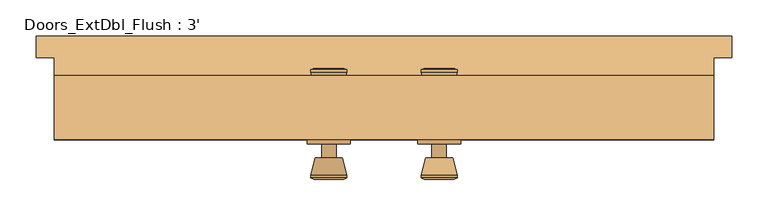
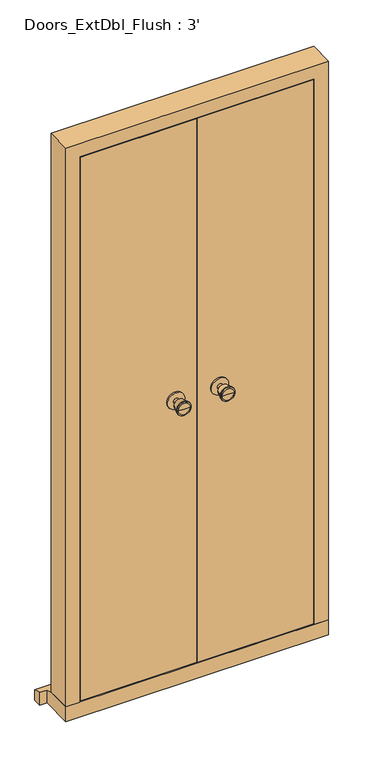
"""IFC4 building model written with IfcOpenShell, lengths in millimetres: door geometry, Doors_ExtDbl_Flush : 3'."""

from ifc_helpers import new_model, si_unit, point, frame, frame_2d, origin, place, context, project, spatial, polyline, circle_curve, trimmed, segment, composite_curve, outline, extrude, faceted_brep, source, transform, mapped, element, save
from ifc_brep_helpers import plane_surface, cylinder_surface, revolved_surface, advanced_brep


def doors_extdbl_flush_3_1e4ff7a8(model_context):
    return source(origin(), model_context, "Body", "SolidModel", [
        advanced_brep(
        [(-76.5, -33.132, 1050.0), (-66.5, -33.132, 1050.0), (-86.5, -33.132, 1050.0), (-96.9758676, -82.132, 1050.0), (-56.0241324, -82.132, 1050.0), (-76.5, -82.132, 1050.0), (-101.5, -80.3041319, 1050.0), (-51.5, -80.3041319, 1050.0), (-101.5, -76.8404537, 1050.0), (-51.5, -76.8404537, 1050.0), (-95.136236, -52.132, 1050.0), (-57.863764, -52.132, 1050.0), (-86.5, -52.132, 1050.0), (-66.5, -52.132, 1050.0)],
        [
            (0, 1),
            (1, 2, circle_curve(frame((-76.5, -33.132, 1050.0), z_axis=(0.0, 1.0, 0.0), x_axis=(1.0, 0.0, 0.0)), 10.0)),
            (2, 0),
            (2, 1, circle_curve(frame((-76.5, -33.132, 1050.0), z_axis=(0.0, 1.0, 0.0), x_axis=(1.0, 0.0, 0.0)), 10.0)),
            (3, 4, circle_curve(frame((-76.5, -82.132, 1050.0), z_axis=(0.0, -1.0, 0.0), x_axis=(1.0, 0.0, 0.0)), 20.4758676)),
            (4, 5),
            (5, 3),
            (4, 3, circle_curve(frame((-76.5, -82.132, 1050.0), z_axis=(0.0, -1.0, 0.0), x_axis=(1.0, 0.0, 0.0)), 20.4758676)),
            (6, 7, circle_curve(frame((-76.5, -80.3041319, 1050.0), z_axis=(0.0, -1.0, 0.0), x_axis=(1.0, 0.0, 0.0)), 25.0)),
            (7, 4),
            (3, 6),
            (7, 6, circle_curve(frame((-76.5, -80.3041319, 1050.0), z_axis=(0.0, -1.0, 0.0), x_axis=(1.0, 0.0, 0.0)), 25.0)),
            (8, 9, circle_curve(frame((-76.5, -76.8404537, 1050.0), z_axis=(0.0, -1.0, 0.0), x_axis=(1.0, 0.0, 0.0)), 25.0)),
            (9, 7),
            (6, 8),
            (9, 8, circle_curve(frame((-76.5, -76.8404537, 1050.0), z_axis=(0.0, -1.0, 0.0), x_axis=(1.0, 0.0, 0.0)), 25.0)),
            (10, 11, circle_curve(frame((-76.5, -52.132, 1050.0), z_axis=(0.0, -1.0, 0.0), x_axis=(1.0, 0.0, 0.0)), 18.636236)),
            (11, 9),
            (8, 10),
            (11, 10, circle_curve(frame((-76.5, -52.132, 1050.0), z_axis=(0.0, -1.0, 0.0), x_axis=(1.0, 0.0, 0.0)), 18.636236)),
            (12, 13, circle_curve(frame((-76.5, -52.132, 1050.0), z_axis=(0.0, -1.0, 0.0), x_axis=(1.0, 0.0, 0.0)), 10.0)),
            (13, 11),
            (10, 12),
            (13, 12, circle_curve(frame((-76.5, -52.132, 1050.0), z_axis=(0.0, -1.0, 0.0), x_axis=(1.0, 0.0, 0.0)), 10.0)),
            (1, 13),
            (12, 2),
        ],
        [
            plane_surface(frame((-76.5, -33.132, 1050.0), z_axis=(0.0, 1.0, 0.0), x_axis=(1.0, 0.0, 0.0))),
            plane_surface(frame((-76.5, -82.132, 1050.0), z_axis=(0.0, -1.0, 0.0), x_axis=(1.0, 0.0, 0.0))),
            revolved_surface(polyline([(-56.0241324, -82.132, 1050.0), (-51.5, -80.3041319, 1050.0)]), (-76.5, -33.132, 1050.0), (0.0, 1.0, 0.0)),
            cylinder_surface(frame((-76.5, -33.132, 1050.0), z_axis=(0.0, 1.0, 0.0), x_axis=(1.0, 0.0, 0.0)), 25.0),
            revolved_surface(polyline([(-51.5, -76.8404537, 1050.0), (-57.863764, -52.132, 1050.0)]), (-76.5, -33.132, 1050.0), (0.0, 1.0, 0.0)),
            plane_surface(frame((-76.5, -52.132, 1050.0), z_axis=(0.0, 1.0, 0.0), x_axis=(1.0, 0.0, 0.0))),
            cylinder_surface(frame((-76.5, -33.132, 1050.0), z_axis=(0.0, 1.0, 0.0), x_axis=(1.0, 0.0, 0.0)), 10.0),
        ],
        [
            (0, [[1, 2, 3]]),
            (0, [[-3, 4, -1]]),
            (1, [[5, 6, 7]]),
            (1, [[8, -7, -6]]),
            (2, [[9, 10, -5, 11]]),
            (2, [[12, -11, -8, -10]]),
            (3, [[13, 14, -9, 15]]),
            (3, [[16, -15, -12, -14]]),
            (4, [[17, 18, -13, 19]]),
            (4, [[20, -19, -16, -18]]),
            (5, [[21, 22, -17, 23]]),
            (5, [[24, -23, -20, -22]]),
            (6, [[-2, 25, -21, 26]]),
            (6, [[-4, -26, -24, -25]]),
        ],
    ),
        extrude(outline(composite_curve([segment(trimmed(circle_curve(frame_2d((1050.0, -76.5)), 30.0), [point((1050.0, -46.5))], [point((1050.0, -106.5))], False, "CARTESIAN"), True, "CONTINUOUS"), segment(trimmed(circle_curve(frame_2d((1050.0, -76.5)), 30.0), [point((1050.0, -106.5))], [point((1050.0, -46.5))], False, "CARTESIAN"), True, "CONTINUOUS")], self_intersect=False)), frame((0.0, -33.132, 0.0), z_axis=(0.0, 1.0, 0.0), x_axis=(0.0, 0.0, 1.0)), (0.0, 0.0, 1.0), 6.0),
        advanced_brep(
        [(-76.5, 22.868, 1050.0), (-86.5, 22.868, 1050.0), (-66.5, 22.868, 1050.0), (-96.9758676, 71.868, 1050.0), (-76.5, 71.868, 1050.0), (-56.0241324, 71.868, 1050.0), (-101.5, 70.0401319, 1050.0), (-51.5, 70.0401319, 1050.0), (-101.5, 66.5764537, 1050.0), (-51.5, 66.5764537, 1050.0), (-95.136236, 41.868, 1050.0), (-57.863764, 41.868, 1050.0), (-86.5, 41.868, 1050.0), (-66.5, 41.868, 1050.0)],
        [
            (0, 1),
            (1, 2, circle_curve(frame((-76.5, 22.868, 1050.0), z_axis=(0.0, -1.0, 0.0), x_axis=(1.0, 0.0, 0.0)), 10.0)),
            (2, 0),
            (2, 1, circle_curve(frame((-76.5, 22.868, 1050.0), z_axis=(0.0, -1.0, 0.0), x_axis=(1.0, 0.0, 0.0)), 10.0)),
            (3, 4),
            (4, 5),
            (5, 3, circle_curve(frame((-76.5, 71.868, 1050.0), z_axis=(0.0, 1.0, 0.0), x_axis=(1.0, 0.0, 0.0)), 20.4758676)),
            (3, 5, circle_curve(frame((-76.5, 71.868, 1050.0), z_axis=(0.0, 1.0, 0.0), x_axis=(1.0, 0.0, 0.0)), 20.4758676)),
            (6, 3),
            (5, 7),
            (7, 6, circle_curve(frame((-76.5, 70.0401319, 1050.0), z_axis=(0.0, 1.0, 0.0), x_axis=(1.0, 0.0, 0.0)), 25.0)),
            (6, 7, circle_curve(frame((-76.5, 70.0401319, 1050.0), z_axis=(0.0, 1.0, 0.0), x_axis=(1.0, 0.0, 0.0)), 25.0)),
            (8, 6),
            (7, 9),
            (9, 8, circle_curve(frame((-76.5, 66.5764537, 1050.0), z_axis=(0.0, 1.0, 0.0), x_axis=(1.0, 0.0, 0.0)), 25.0)),
            (8, 9, circle_curve(frame((-76.5, 66.5764537, 1050.0), z_axis=(0.0, 1.0, 0.0), x_axis=(1.0, 0.0, 0.0)), 25.0)),
            (10, 8),
            (9, 11),
            (11, 10, circle_curve(frame((-76.5, 41.868, 1050.0), z_axis=(0.0, 1.0, 0.0), x_axis=(1.0, 0.0, 0.0)), 18.636236)),
            (10, 11, circle_curve(frame((-76.5, 41.868, 1050.0), z_axis=(0.0, 1.0, 0.0), x_axis=(1.0, 0.0, 0.0)), 18.636236)),
            (12, 10),
            (11, 13),
            (13, 12, circle_curve(frame((-76.5, 41.868, 1050.0), z_axis=(0.0, 1.0, 0.0), x_axis=(1.0, 0.0, 0.0)), 10.0)),
            (12, 13, circle_curve(frame((-76.5, 41.868, 1050.0), z_axis=(0.0, 1.0, 0.0), x_axis=(1.0, 0.0, 0.0)), 10.0)),
            (1, 12),
            (13, 2),
        ],
        [
            plane_surface(frame((-76.5, 22.868, 1050.0), z_axis=(0.0, -1.0, 0.0), x_axis=(1.0, 0.0, 0.0))),
            plane_surface(frame((-76.5, 71.868, 1050.0), z_axis=(0.0, 1.0, 0.0), x_axis=(1.0, 0.0, 0.0))),
            revolved_surface(polyline([(-56.0241324, 71.868, 1050.0), (-51.5, 70.0401319, 1050.0)]), (-76.5, 22.868, 1050.0), (0.0, -1.0, 0.0)),
            cylinder_surface(frame((-76.5, 22.868, 1050.0), z_axis=(0.0, -1.0, 0.0), x_axis=(1.0, 0.0, 0.0)), 25.0),
            revolved_surface(polyline([(-51.5, 66.5764537, 1050.0), (-57.863764, 41.868, 1050.0)]), (-76.5, 22.868, 1050.0), (0.0, -1.0, 0.0)),
            plane_surface(frame((-76.5, 41.868, 1050.0), z_axis=(0.0, -1.0, 0.0), x_axis=(1.0, 0.0, 0.0))),
            cylinder_surface(frame((-76.5, 22.868, 1050.0), z_axis=(0.0, -1.0, 0.0), x_axis=(1.0, 0.0, 0.0)), 10.0),
        ],
        [
            (0, [[1, 2, 3]]),
            (0, [[-3, 4, -1]]),
            (1, [[5, 6, 7]]),
            (1, [[-6, -5, 8]]),
            (2, [[9, -7, 10, 11]]),
            (2, [[-10, -8, -9, 12]]),
            (3, [[13, -11, 14, 15]]),
            (3, [[-14, -12, -13, 16]]),
            (4, [[17, -15, 18, 19]]),
            (4, [[-18, -16, -17, 20]]),
            (5, [[21, -19, 22, 23]]),
            (5, [[-22, -20, -21, 24]]),
            (6, [[25, -23, 26, -2]]),
            (6, [[-26, -24, -25, -4]]),
        ],
    ),
        extrude(outline(composite_curve([segment(trimmed(circle_curve(frame_2d((1050.0, -76.5)), 30.0), [point((1050.0, -46.5))], [point((1050.0, -106.5))], False, "CARTESIAN"), True, "CONTINUOUS"), segment(trimmed(circle_curve(frame_2d((1050.0, -76.5)), 30.0), [point((1050.0, -106.5))], [point((1050.0, -46.5))], False, "CARTESIAN"), True, "CONTINUOUS")], self_intersect=False)), frame((0.0, 16.868, 0.0), z_axis=(0.0, 1.0, 0.0), x_axis=(0.0, 0.0, 1.0)), (0.0, 0.0, 1.0), 6.0),
        advanced_brep(
        [(76.5, -33.132, 1050.0), (86.5, -33.132, 1050.0), (66.5, -33.132, 1050.0), (96.9758676, -82.132, 1050.0), (76.5, -82.132, 1050.0), (56.0241324, -82.132, 1050.0), (101.5, -80.3041319, 1050.0), (51.5, -80.3041319, 1050.0), (101.5, -76.8404537, 1050.0), (51.5, -76.8404537, 1050.0), (95.136236, -52.132, 1050.0), (57.863764, -52.132, 1050.0), (86.5, -52.132, 1050.0), (66.5, -52.132, 1050.0)],
        [
            (0, 1),
            (1, 2, circle_curve(frame((76.5, -33.132, 1050.0), z_axis=(0.0, 1.0, 0.0), x_axis=(-1.0, 0.0, 0.0)), 10.0)),
            (2, 0),
            (2, 1, circle_curve(frame((76.5, -33.132, 1050.0), z_axis=(0.0, 1.0, 0.0), x_axis=(-1.0, 0.0, 0.0)), 10.0)),
            (3, 4),
            (4, 5),
            (5, 3, circle_curve(frame((76.5, -82.132, 1050.0), z_axis=(0.0, -1.0, 0.0), x_axis=(-1.0, 0.0, 0.0)), 20.4758676)),
            (3, 5, circle_curve(frame((76.5, -82.132, 1050.0), z_axis=(0.0, -1.0, 0.0), x_axis=(-1.0, 0.0, 0.0)), 20.4758676)),
            (6, 3),
            (5, 7),
            (7, 6, circle_curve(frame((76.5, -80.3041319, 1050.0), z_axis=(0.0, -1.0, 0.0), x_axis=(-1.0, 0.0, 0.0)), 25.0)),
            (6, 7, circle_curve(frame((76.5, -80.3041319, 1050.0), z_axis=(0.0, -1.0, 0.0), x_axis=(-1.0, 0.0, 0.0)), 25.0)),
            (8, 6),
            (7, 9),
            (9, 8, circle_curve(frame((76.5, -76.8404537, 1050.0), z_axis=(0.0, -1.0, 0.0), x_axis=(-1.0, 0.0, 0.0)), 25.0)),
            (8, 9, circle_curve(frame((76.5, -76.8404537, 1050.0), z_axis=(0.0, -1.0, 0.0), x_axis=(-1.0, 0.0, 0.0)), 25.0)),
            (10, 8),
            (9, 11),
            (11, 10, circle_curve(frame((76.5, -52.132, 1050.0), z_axis=(0.0, -1.0, 0.0), x_axis=(-1.0, 0.0, 0.0)), 18.636236)),
            (10, 11, circle_curve(frame((76.5, -52.132, 1050.0), z_axis=(0.0, -1.0, 0.0), x_axis=(-1.0, 0.0, 0.0)), 18.636236)),
            (12, 10),
            (11, 13),
            (13, 12, circle_curve(frame((76.5, -52.132, 1050.0), z_axis=(0.0, -1.0, 0.0), x_axis=(-1.0, 0.0, 0.0)), 10.0)),
            (12, 13, circle_curve(frame((76.5, -52.132, 1050.0), z_axis=(0.0, -1.0, 0.0), x_axis=(-1.0, 0.0, 0.0)), 10.0)),
            (1, 12),
            (13, 2),
        ],
        [
            plane_surface(frame((76.5, -33.132, 1050.0), z_axis=(0.0, 1.0, 0.0), x_axis=(-1.0, 0.0, 0.0))),
            plane_surface(frame((76.5, -82.132, 1050.0), z_axis=(0.0, -1.0, 0.0), x_axis=(-1.0, 0.0, 0.0))),
            revolved_surface(polyline([(56.0241324, -82.132, 1050.0), (51.5, -80.3041319, 1050.0)]), (76.5, -33.132, 1050.0), (0.0, 1.0, 0.0)),
            cylinder_surface(frame((76.5, -33.132, 1050.0), z_axis=(0.0, 1.0, 0.0), x_axis=(-1.0, 0.0, 0.0)), 25.0),
            revolved_surface(polyline([(51.5, -76.8404537, 1050.0), (57.863764, -52.132, 1050.0)]), (76.5, -33.132, 1050.0), (0.0, 1.0, 0.0)),
            plane_surface(frame((76.5, -52.132, 1050.0), z_axis=(0.0, 1.0, 0.0), x_axis=(-1.0, 0.0, 0.0))),
            cylinder_surface(frame((76.5, -33.132, 1050.0), z_axis=(0.0, 1.0, 0.0), x_axis=(-1.0, 0.0, 0.0)), 10.0),
        ],
        [
            (0, [[1, 2, 3]]),
            (0, [[-3, 4, -1]]),
            (1, [[5, 6, 7]]),
            (1, [[-6, -5, 8]]),
            (2, [[9, -7, 10, 11]]),
            (2, [[-10, -8, -9, 12]]),
            (3, [[13, -11, 14, 15]]),
            (3, [[-14, -12, -13, 16]]),
            (4, [[17, -15, 18, 19]]),
            (4, [[-18, -16, -17, 20]]),
            (5, [[21, -19, 22, 23]]),
            (5, [[-22, -20, -21, 24]]),
            (6, [[25, -23, 26, -2]]),
            (6, [[-26, -24, -25, -4]]),
        ],
    ),
        extrude(outline(composite_curve([segment(trimmed(circle_curve(frame_2d((1050.0, 76.5)), 30.0), [point((1050.0, 46.5))], [point((1050.0, 106.5))], False, "CARTESIAN"), True, "CONTINUOUS"), segment(trimmed(circle_curve(frame_2d((1050.0, 76.5)), 30.0), [point((1050.0, 106.5))], [point((1050.0, 46.5))], False, "CARTESIAN"), True, "CONTINUOUS")], self_intersect=False)), frame((0.0, -33.132, 0.0), z_axis=(0.0, 1.0, 0.0), x_axis=(0.0, 0.0, 1.0)), (0.0, 0.0, 1.0), 6.0),
        advanced_brep(
        [(76.5, 22.868, 1050.0), (66.5, 22.868, 1050.0), (86.5, 22.868, 1050.0), (96.9758676, 71.868, 1050.0), (56.0241324, 71.868, 1050.0), (76.5, 71.868, 1050.0), (101.5, 70.0401319, 1050.0), (51.5, 70.0401319, 1050.0), (101.5, 66.5764537, 1050.0), (51.5, 66.5764537, 1050.0), (95.136236, 41.868, 1050.0), (57.863764, 41.868, 1050.0), (86.5, 41.868, 1050.0), (66.5, 41.868, 1050.0)],
        [
            (0, 1),
            (1, 2, circle_curve(frame((76.5, 22.868, 1050.0), z_axis=(0.0, -1.0, 0.0), x_axis=(-1.0, 0.0, 0.0)), 10.0)),
            (2, 0),
            (2, 1, circle_curve(frame((76.5, 22.868, 1050.0), z_axis=(0.0, -1.0, 0.0), x_axis=(-1.0, 0.0, 0.0)), 10.0)),
            (3, 4, circle_curve(frame((76.5, 71.868, 1050.0), z_axis=(0.0, 1.0, 0.0), x_axis=(-1.0, 0.0, 0.0)), 20.4758676)),
            (4, 5),
            (5, 3),
            (4, 3, circle_curve(frame((76.5, 71.868, 1050.0), z_axis=(0.0, 1.0, 0.0), x_axis=(-1.0, 0.0, 0.0)), 20.4758676)),
            (6, 7, circle_curve(frame((76.5, 70.0401319, 1050.0), z_axis=(0.0, 1.0, 0.0), x_axis=(-1.0, 0.0, 0.0)), 25.0)),
            (7, 4),
            (3, 6),
            (7, 6, circle_curve(frame((76.5, 70.0401319, 1050.0), z_axis=(0.0, 1.0, 0.0), x_axis=(-1.0, 0.0, 0.0)), 25.0)),
            (8, 9, circle_curve(frame((76.5, 66.5764537, 1050.0), z_axis=(0.0, 1.0, 0.0), x_axis=(-1.0, 0.0, 0.0)), 25.0)),
            (9, 7),
            (6, 8),
            (9, 8, circle_curve(frame((76.5, 66.5764537, 1050.0), z_axis=(0.0, 1.0, 0.0), x_axis=(-1.0, 0.0, 0.0)), 25.0)),
            (10, 11, circle_curve(frame((76.5, 41.868, 1050.0), z_axis=(0.0, 1.0, 0.0), x_axis=(-1.0, 0.0, 0.0)), 18.636236)),
            (11, 9),
            (8, 10),
            (11, 10, circle_curve(frame((76.5, 41.868, 1050.0), z_axis=(0.0, 1.0, 0.0), x_axis=(-1.0, 0.0, 0.0)), 18.636236)),
            (12, 13, circle_curve(frame((76.5, 41.868, 1050.0), z_axis=(0.0, 1.0, 0.0), x_axis=(-1.0, 0.0, 0.0)), 10.0)),
            (13, 11),
            (10, 12),
            (13, 12, circle_curve(frame((76.5, 41.868, 1050.0), z_axis=(0.0, 1.0, 0.0), x_axis=(-1.0, 0.0, 0.0)), 10.0)),
            (1, 13),
            (12, 2),
        ],
        [
            plane_surface(frame((76.5, 22.868, 1050.0), z_axis=(0.0, -1.0, 0.0), x_axis=(-1.0, 0.0, 0.0))),
            plane_surface(frame((76.5, 71.868, 1050.0), z_axis=(0.0, 1.0, 0.0), x_axis=(-1.0, 0.0, 0.0))),
            revolved_surface(polyline([(56.0241324, 71.868, 1050.0), (51.5, 70.0401319, 1050.0)]), (76.5, 22.868, 1050.0), (0.0, -1.0, 0.0)),
            cylinder_surface(frame((76.5, 22.868, 1050.0), z_axis=(0.0, -1.0, 0.0), x_axis=(-1.0, 0.0, 0.0)), 25.0),
            revolved_surface(polyline([(51.5, 66.5764537, 1050.0), (57.863764, 41.868, 1050.0)]), (76.5, 22.868, 1050.0), (0.0, -1.0, 0.0)),
            plane_surface(frame((76.5, 41.868, 1050.0), z_axis=(0.0, -1.0, 0.0), x_axis=(-1.0, 0.0, 0.0))),
            cylinder_surface(frame((76.5, 22.868, 1050.0), z_axis=(0.0, -1.0, 0.0), x_axis=(-1.0, 0.0, 0.0)), 10.0),
        ],
        [
            (0, [[1, 2, 3]]),
            (0, [[-3, 4, -1]]),
            (1, [[5, 6, 7]]),
            (1, [[8, -7, -6]]),
            (2, [[9, 10, -5, 11]]),
            (2, [[12, -11, -8, -10]]),
            (3, [[13, 14, -9, 15]]),
            (3, [[16, -15, -12, -14]]),
            (4, [[17, 18, -13, 19]]),
            (4, [[20, -19, -16, -18]]),
            (5, [[21, 22, -17, 23]]),
            (5, [[24, -23, -20, -22]]),
            (6, [[-2, 25, -21, 26]]),
            (6, [[-4, -26, -24, -25]]),
        ],
    ),
        extrude(outline(composite_curve([segment(trimmed(circle_curve(frame_2d((1050.0, 76.5)), 30.0), [point((1050.0, 46.5))], [point((1050.0, 106.5))], False, "CARTESIAN"), True, "CONTINUOUS"), segment(trimmed(circle_curve(frame_2d((1050.0, 76.5)), 30.0), [point((1050.0, 106.5))], [point((1050.0, 46.5))], False, "CARTESIAN"), True, "CONTINUOUS")], self_intersect=False)), frame((0.0, 16.868, 0.0), z_axis=(0.0, 1.0, 0.0), x_axis=(0.0, 0.0, 1.0)), (0.0, 0.0, 1.0), 6.0),
        faceted_brep([(386.7, 61.868, 54.5), (457.2, 61.868, 54.5), (457.2, -27.132, 54.5), (408.7, -27.132, 54.5), (408.7, 19.868, 54.5), (386.7, 19.868, 54.5), (386.7, 61.868, 2039.5), (-386.7, 61.868, 2039.5), (-386.7, 61.868, 54.5), (-457.2, 61.868, 54.5), (-457.2, 61.868, 2110.0), (457.2, 61.868, 2110.0), (457.2, -27.132, 2110.0), (-457.2, -27.132, 2110.0), (-457.2, -27.132, 54.5), (-408.7, -27.132, 54.5), (-408.7, -27.132, 2061.5), (408.7, -27.132, 2061.5), (408.7, 19.868, 2061.5), (-408.7, 19.868, 2061.5), (-408.7, 19.868, 54.5), (-386.7, 19.868, 54.5), (-386.7, 19.868, 2039.5), (386.7, 19.868, 2039.5)], [[[0, 1, 2, 3, 4, 5]], [[1, 0, 6, 7, 8, 9, 10, 11]], [[2, 1, 11, 12]], [[3, 2, 12, 13, 14, 15, 16, 17]], [[4, 3, 17, 18]], [[5, 4, 18, 19, 20, 21, 22, 23]], [[0, 5, 23, 6]], [[7, 22, 21, 8]], [[8, 21, 20, 15, 14, 9]], [[13, 10, 9, 14]], [[19, 16, 15, 20]], [[12, 11, 10, 13]], [[18, 17, 16, 19]], [[6, 23, 22, 7]]]),
        faceted_brep([(482.2, 116.868, 0.0), (482.2, 116.868, 38.5947221), (482.2, 86.868, 47.2703282), (482.2, 86.868, 0.0), (-482.2, 116.868, 38.5947221), (-482.2, 116.868, 0.0), (-482.2, 86.868, 0.0), (-482.2, 86.868, 47.2703282), (457.2, 86.868, 0.0), (457.2, -27.132, 0.0), (-457.2, -27.132, 0.0), (-457.2, 86.868, 0.0), (-457.2, 86.868, 47.2703282), (-457.2, 61.868, 54.5), (457.2, 61.868, 54.5), (457.2, 86.868, 47.2703282), (-457.2, -27.132, 54.5), (457.2, -27.132, 54.5)], [[[0, 1, 2, 3]], [[4, 5, 6, 7]], [[5, 0, 3, 8, 9, 10, 11, 6]], [[1, 0, 5, 4]], [[1, 4, 7, 12, 13, 14, 15, 2]], [[13, 16, 17, 14]], [[16, 10, 9, 17]], [[12, 11, 10, 16, 13]], [[11, 12, 7, 6]], [[8, 15, 14, 17, 9]], [[15, 8, 3, 2]]]),
        extrude(outline(polyline([(405.7, -27.132), (1.5, -27.132), (1.5, 16.868), (405.7, 16.868), (405.7, -27.132)])), frame((0.0, 0.0, 58.5), z_axis=(0.0, 0.0, 1.0), x_axis=(1.0, 0.0, 0.0)), (0.0, 0.0, 1.0), 2000.0),
        extrude(outline(polyline([(-1.5, -27.132), (-405.7, -27.132), (-405.7, 16.868), (-1.5, 16.868), (-1.5, -27.132)])), frame((0.0, 0.0, 58.5), z_axis=(0.0, 0.0, 1.0), x_axis=(1.0, 0.0, 0.0)), (0.0, 0.0, 1.0), 2000.0),
    ])


if __name__ == "__main__":
    model = new_model("IFC4")
    model_context = context("Model", 3, world=origin())
    ifc_project = project(units=[si_unit("LENGTHUNIT", "METRE", prefix="MILLI")], contexts=[model_context])
    site = spatial("IfcSite", under=ifc_project)
    building = spatial("IfcBuilding", under=site)
    placement = place(None, origin())
    doors_extdbl_flush_3_shape = doors_extdbl_flush_3_1e4ff7a8(model_context)
    element("IfcDoor", 1, ObjectType="Doors_ExtDbl_Flush : 3'", at=placement, inside=building, context=model_context, shape_type="MappedRepresentation", body=[
        mapped(doors_extdbl_flush_3_shape, transform((0.0, 0.0, 0.0), x_axis=(1.0, 0.0, 0.0), y_axis=(0.0, 1.0, 0.0), z_axis=(0.0, 0.0, 1.0))),
    ])
    save(model, "model.ifc")

# Revit data of these elements
# Type "Doors_ExtDbl_Flush : 3'"
#   Type Mark = "55"
#   Type Comments = "External Double"
#   Operation = "DoubleDoorSingleSwing"
#   Keynote = "L20"
#   Analytic Construction = "Metal"
#   Wrap Layers (Ext) from Ext = 0.336286 ft
#   Wrap Layers (Int) from Ext = 0.582349 ft
#   Thickness = 0.144357 ft
#   Rough Width = 3.0 ft
#   Rough Height = 6.922572 ft
#   O/A Frame Width = 0.209974 ft
#   Heat Transfer Coefficient (U) = 3.7021 W/(m²·K)
#   Handle Z Distance = 3.444882 ft
#   FrameWidth = 0.137795 ft
#   FrameOffset - External = 0.082021 ft
#   FrameDepth = 0.291995 ft
#   Door Panel Width = 1.326115 ft
#   Door Panel Thickness = 0.144357 ft
#   Door Panel Height = 6.56168 ft
#   Cill Thickness = 0.178806 ft
#   Cill Projection = 0.098425 ft
#   Handle X Distance = 0.246063 ft
#   Height = 6.922572 ft
#   Structural Tolerance = 0.021325 ft
#   Tolerance = 0.009843 ft
#   Undercut = 0.013123 ft
#   Width = 3.0 ft
#   Cill Extension = 0.082021 ft
#   Cavity Closer Width = 0.164042 ft
#   Cavity Closer Offset from Ext = 0.336286 ft
#   Cavity Closer Depth = 0.278871 ft
#   Vis - Ironmongery = yes
#   Vis - Cavity Closers = yes
#   Function = 1
#   Material Door = Door - Panel
#   Material Frame = Door - Frame/Mullion
#   Material Ironmongery = Door - Handle
#   Visual Light Transmittance = 0
#   Thermal Resistance (R) = 0
#   Solar Heat Gain Coefficient = 0
#   Wall Closure = (empty or 0)
# Element 1 (IfcDoor, "Doors_ExtDbl_Flush : 3'")
#   Materials on its faces: "Door - Handle", "Door - Frame/Mullion", "Door - Panel"
# Materials
#   "Door - Panel": class "Wood", colour RGB 210 159 95, transparency 0, Keynote = "L20", Cost = 0
#   "Door - Frame/Mullion": class "Wood", colour RGB 212 179 113, transparency 0, Keynote = "L20", Cost = 0
#   "Door - Handle": colour RGB 0 0 0, transparency 0, Keynote = "P21", Cost = 0
